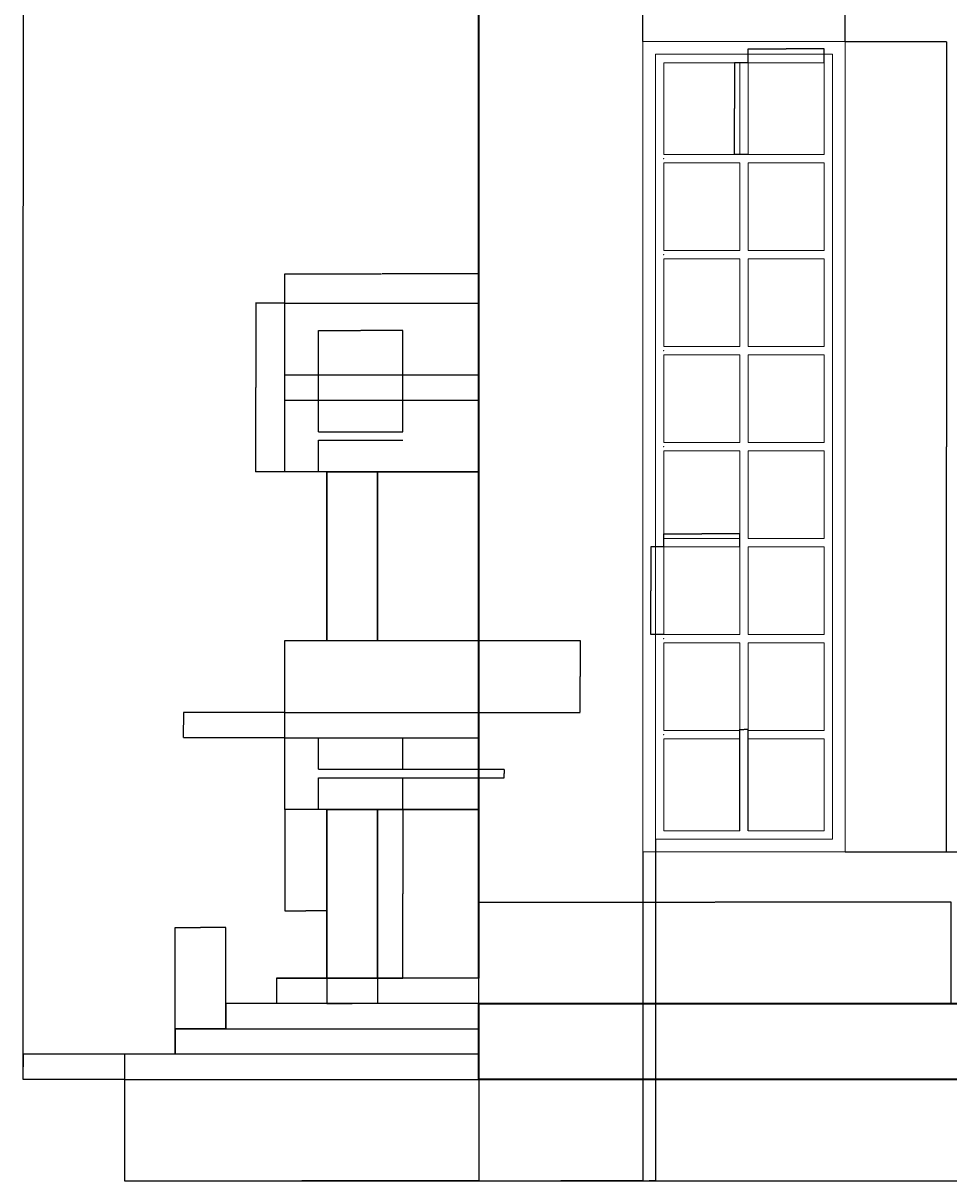
# Model space of a CAD drawing. Units: millimetres. Extents: x 54 to 12356, y 76 to 11627.
# Tile 1 of 2: x 54 to 5541, y 76 to 6935. Entities that reach past the tile are written whole.
import ezdxf

# ---------------------------------------------------------------- set-up
doc = ezdxf.new("R2010")
doc.units = ezdxf.units.MM
for name, color, linetype, lineweight in [('A-ANNO-DIMS', 2, 'Continuous', 18), ('A-COLS', 7, 'Continuous', 30), ('A-FLOR', 7, 'Continuous', 25), ('A-FLOR-STRS', 7, 'Continuous', 25), ('A-GLAZ', 4, 'Continuous', 18), ('A-GLAZ-LAYO', 8, 'Continuous', 13), ('A-WALL', 7, 'Continuous', 35), ('S-FNDN', 7, 'Continuous', 35)]:
    doc.layers.add(name, color=color, linetype=linetype, lineweight=lineweight)
doc.styles.get("Standard").update_dxf_attribs({"font": 'arial.ttf'})
doc.dimstyles.get("Standard").update_dxf_attribs({"dimtxt": 0.18, "dimasz": 0.18, "dimexe": 0.18, "dimexo": 0.0625, "dimgap": 0.09, "dimtad": 0, "dimtih": 1, "dimtoh": 1, "dimdec": 4, "dimzin": 0, "dimdsep": 46, "dimtxsty": 'Standard', "dimcen": 0.09, "dimadec": 0, "dimazin": 0, "dimtfac": 1, "dimtdec": 4, "dimtofl": 0, "dimtmove": 0, "dimatfit": 3, "dimfxl": 1, "dimtolj": 1, "dimtzin": 0, "dimarcsym": 0})

# ---------------------------------------------------------------- blocks, each defined once
blk = doc.blocks.new('STAIR-GLAZ-LITE-INTERMEDIATE')
for p, q in [((0.0003419131726332, 518.7501830437077), (450.0003419131708, 518.7501830437077)), ((0.0003419131726332, 0.0001830437076933), (0.000341913173088, 518.7501830437077)), ((450.0003419131717, 518.7501830437077), (450.0003419131726, 0.0001830437076933)), ((0.0003419131726332, 0.0001830437076933), (450.0003419131717, 0.0001830437076933))]:
    blk.add_line(p, q)
blk = doc.blocks.new('STAIR-GLAZ-LITE-END')
for p, q in [((0.0003419131726332, 543.7501830437077), (0.0003419131717237, 0.0001830437067838)), ((0.0003419131735427, 543.7501830437077), (450.0003419131726, 543.7501830437077)), ((450.0003419131726, 543.7501830437077), (450.0003419131726, 0.0001830437067838)), ((0.0003419131726332, 0.0001830437076933), (450.0003419131726, 0.0001830437076933))]:
    blk.add_line(p, q)
blk = doc.blocks.new('PORCH-COLUMN-300')
for p, q in [((0.0002773238852569, 0.0003573361398139), (0.0002773238852569, 1000.00035733614)), ((300.0002773238853, 0.0003573361398139), (300.0002773238853, 1000.00035733614))]:
    blk.add_line(p, q)
blk = doc.blocks.new('PORCH-FASCIA-1150')
for p, q in [((0.0002773238852569, 1000.00035733614), (1150.000277323885, 1000.00035733614)), ((0.0002773238852569, 575.00035733614), (0.0002773238852569, 1000.00035733614)), ((0.0002773238852569, 575.00035733614), (1150.000277323885, 575.00035733614)), ((0.0002773238852569, 425.00035733614), (0.0002773238852569, 575.00035733614)), ((0.0002773238852569, 0.0003573361400413), (0.0002773238852569, 425.00035733614)), ((0.0002773238852569, 425.00035733614), (1150.000277323885, 425.00035733614)), ((250.0002773238853, 0.0003573361400413), (0.0002773238852569, 0.0003573361400413)), ((250.0002773238853, 0.0003573361400413), (1150.000277323885, 0.0003573361400413)), ((1150.000277323885, 0.0003573361400413), (250.0002773238853, 0.0003573361400413))]:
    blk.add_line(p, q)
blk = doc.blocks.new('*D7')
at = {"layer": 'A-ANNO-DIMS', "color": 0, "lineweight": -2, "transparency": 16777216}
for p, q in [((3851.677841913175, 3831.536183043709), (3773.747841913177, 3831.536183043709)), ((3773.927841913176, 3831.356183043709), (3773.927841913176, 3572.343086181499)), ((3773.927841913176, 3312.966183043709), (3773.927841913176, 3571.97927990592)), ((3851.677841913175, 3312.786183043709), (3773.747841913177, 3312.786183043709))]:
    blk.add_line(p, q, dxfattribs=at)
at = {"layer": 'A-ANNO-DIMS', "color": 0, "transparency": 16777216}
for points in [[(3773.897841913176, 3831.356183043709), (3773.957841913177, 3831.356183043709), (3773.927841913176, 3831.536183043709)], [(3773.897841913176, 3312.966183043709), (3773.957841913177, 3312.966183043709), (3773.927841913176, 3312.786183043709)]]:
    blk.add_solid(points, dxfattribs=at)
at = {"layer": 'Defpoints', "color": 0, "transparency": 16777216}
for p in [(3851.740341913174, 3831.536183043709), (3773.927841913176, 3312.786183043709), (3851.740341913174, 3312.786183043709)]:
    blk.add_point(p, dxfattribs=at)
at = {"layer": 'A-ANNO-DIMS', "color": 0, "transparency": 16777216, "insert": (3773.927841913176, 3572.161183043707), "char_height": 0.18, "attachment_point": 5}
blk.add_mtext('\\A1;INTERMEDIATE LITE 519 TYP.', dxfattribs=at)
blk = doc.blocks.new('*D8')
at = {"layer": 'A-ANNO-DIMS', "color": 0, "lineweight": -2, "transparency": 16777216}
for p, q in [((3851.740341913173, 3831.598683043708), (3851.740341913173, 3909.528683043708)), ((3851.920341913173, 3909.348683043707), (4076.138704805396, 3909.348683043707)), ((4301.560341913172, 3909.348683043707), (4077.341979020949, 3909.348683043707)), ((4301.740341913173, 3831.598683043708), (4301.740341913173, 3909.528683043708))]:
    blk.add_line(p, q, dxfattribs=at)
at = {"layer": 'A-ANNO-DIMS', "color": 0, "transparency": 16777216}
for points in [[(3851.920341913173, 3909.378683043708), (3851.920341913173, 3909.318683043707), (3851.740341913173, 3909.348683043707)], [(4301.560341913172, 3909.378683043708), (4301.560341913172, 3909.318683043707), (4301.740341913173, 3909.348683043707)]]:
    blk.add_solid(points, dxfattribs=at)
at = {"layer": 'Defpoints', "color": 0, "transparency": 16777216}
for p in [(3851.740341913173, 3909.348683043707), (3851.740341913173, 3831.536183043708), (4301.740341913173, 3831.536183043708)]:
    blk.add_point(p, dxfattribs=at)
at = {"layer": 'A-ANNO-DIMS', "color": 0, "transparency": 16777216, "insert": (4076.740341913172, 3909.348683043707), "char_height": 0.18, "attachment_point": 5}
blk.add_mtext('\\A1;450 TYP.', dxfattribs=at)
blk = doc.blocks.new('*D9')
at = {"layer": 'A-ANNO-DIMS', "color": 0, "lineweight": -2, "transparency": 16777216}
for p, q in [((4351.677841913173, 6700.286183043711), (4269.997841913174, 6700.286183043711)), ((4270.177841913175, 6700.106183043711), (4270.177841913175, 6428.592717832252)), ((4270.177841913175, 6156.716183043711), (4270.177841913175, 6428.229648255172)), ((4351.677841913173, 6156.53618304371), (4269.997841913174, 6156.53618304371))]:
    blk.add_line(p, q, dxfattribs=at)
at = {"layer": 'A-ANNO-DIMS', "color": 0, "transparency": 16777216}
for points in [[(4270.147841913175, 6700.106183043711), (4270.207841913175, 6700.106183043711), (4270.177841913175, 6700.286183043711)], [(4270.147841913175, 6156.716183043711), (4270.207841913175, 6156.716183043711), (4270.177841913175, 6156.53618304371)]]:
    blk.add_solid(points, dxfattribs=at)
at = {"layer": 'Defpoints', "color": 0, "transparency": 16777216}
for p in [(4270.177841913175, 6700.286183043711), (4351.740341913173, 6700.286183043711), (4351.740341913173, 6156.53618304371)]:
    blk.add_point(p, dxfattribs=at)
at = {"layer": 'A-ANNO-DIMS', "color": 0, "transparency": 16777216, "insert": (4270.177841913176, 6428.411183043708), "char_height": 0.18, "attachment_point": 5}
blk.add_mtext('\\A1;END LITE 544 TYP.', dxfattribs=at)
blk = doc.blocks.new('*D10')
at = {"layer": 'A-ANNO-DIMS', "color": 0, "lineweight": -2, "transparency": 16777216}
for p, q in [((4351.740341913171, 6700.348683043708), (4351.740341913171, 6782.028683043709)), ((4351.920341913172, 6781.848683043708), (4576.138704805394, 6781.848683043708)), ((4801.560341913172, 6781.848683043708), (4577.341979020948, 6781.848683043708)), ((4801.740341913173, 6700.348683043708), (4801.740341913173, 6782.028683043709))]:
    blk.add_line(p, q, dxfattribs=at)
at = {"layer": 'A-ANNO-DIMS', "color": 0, "transparency": 16777216}
for points in [[(4351.920341913172, 6781.878683043707), (4351.920341913172, 6781.818683043709), (4351.740341913171, 6781.848683043708)], [(4801.560341913172, 6781.878683043707), (4801.560341913172, 6781.818683043709), (4801.740341913173, 6781.848683043708)]]:
    blk.add_solid(points, dxfattribs=at)
at = {"layer": 'Defpoints', "color": 0, "transparency": 16777216}
for p in [(4801.740341913173, 6781.848683043708), (4351.740341913171, 6700.286183043708), (4801.740341913173, 6700.286183043708)]:
    blk.add_point(p, dxfattribs=at)
at = {"layer": 'A-ANNO-DIMS', "color": 0, "transparency": 16777216, "insert": (4576.740341913171, 6781.848683043708), "char_height": 0.18, "attachment_point": 5}
blk.add_mtext('\\A1;450 TYP.', dxfattribs=at)
blk = doc.blocks.new('*D15')
at = {"layer": 'A-ANNO-DIMS', "color": 0, "lineweight": -2, "transparency": 16777216}
for p, q in [((2154.993777323886, 2276.423357336141), (2305.111277323887, 2276.423357336141)), ((2304.931277323887, 2276.243357336141), (2304.931277323887, 1776.606488304763)), ((2304.931277323887, 1276.60335733614), (2304.931277323887, 1776.240226367518)), ((2154.993777323886, 1276.42335733614), (2305.111277323887, 1276.42335733614))]:
    blk.add_line(p, q, dxfattribs=at)
at = {"layer": 'A-ANNO-DIMS', "color": 0, "transparency": 16777216}
for points in [[(2304.901277323887, 2276.243357336141), (2304.961277323887, 2276.243357336141), (2304.931277323887, 2276.423357336141)], [(2304.901277323887, 1276.60335733614), (2304.961277323887, 1276.60335733614), (2304.931277323887, 1276.42335733614)]]:
    blk.add_solid(points, dxfattribs=at)
at = {"layer": 'Defpoints', "color": 0, "transparency": 16777216}
for p in [(2154.931277323886, 2276.423357336141), (2304.931277323887, 2276.423357336141), (2154.931277323886, 1276.42335733614)]:
    blk.add_point(p, dxfattribs=at)
at = {"layer": 'A-ANNO-DIMS', "color": 0, "transparency": 16777216, "insert": (2304.931277323887, 1776.423357336139), "char_height": 0.18, "attachment_point": 5}
blk.add_mtext('\\A1;PORCH COLUMN 1000 TYP.', dxfattribs=at)
blk = doc.blocks.new('*D16')
at = {"layer": 'A-ANNO-DIMS', "color": 0, "lineweight": -2, "transparency": 16777216}
for p, q in [((1854.931277323885, 1276.36085733614), (1854.931277323885, 1126.243357336139)), ((2154.931277323886, 1276.36085733614), (2154.931277323886, 1126.243357336139)), ((1855.111277323885, 1126.42335733614), (2004.333323708606, 1126.42335733614)), ((2154.751277323885, 1126.42335733614), (2005.529230939165, 1126.42335733614))]:
    blk.add_line(p, q, dxfattribs=at)
at = {"layer": 'A-ANNO-DIMS', "color": 0, "transparency": 16777216}
for points in [[(1855.111277323885, 1126.453357336139), (1855.111277323885, 1126.39335733614), (1854.931277323885, 1126.42335733614)], [(2154.751277323885, 1126.453357336139), (2154.751277323885, 1126.39335733614), (2154.931277323886, 1126.42335733614)]]:
    blk.add_solid(points, dxfattribs=at)
at = {"layer": 'Defpoints', "color": 0, "transparency": 16777216}
for p in [(1854.931277323885, 1276.42335733614), (2154.931277323886, 1276.42335733614), (2154.931277323886, 1126.42335733614)]:
    blk.add_point(p, dxfattribs=at)
at = {"layer": 'A-ANNO-DIMS', "color": 0, "transparency": 16777216, "insert": (2004.931277323885, 1126.42335733614), "char_height": 0.18, "attachment_point": 5}
blk.add_mtext('\\A1;300 TYP.', dxfattribs=at)
blk = doc.blocks.new('*D17')
at = {"layer": 'A-ANNO-DIMS', "color": 0, "lineweight": -2, "transparency": 16777216}
for p, q in [((1604.931277323885, 5276.48585733614), (1604.931277323885, 5449.10335733614)), ((1605.111277323885, 5448.923357336139), (2178.289790284322, 5448.923357336139)), ((2754.751277323885, 5448.923357336139), (2181.572764363449, 5448.923357336139)), ((2754.931277323886, 5276.48585733614), (2754.931277323886, 5449.10335733614))]:
    blk.add_line(p, q, dxfattribs=at)
at = {"layer": 'A-ANNO-DIMS', "color": 0, "transparency": 16777216}
for points in [[(1605.111277323885, 5448.95335733614), (1605.111277323885, 5448.89335733614), (1604.931277323885, 5448.923357336139)], [(2754.751277323885, 5448.95335733614), (2754.751277323885, 5448.89335733614), (2754.931277323886, 5448.923357336139)]]:
    blk.add_solid(points, dxfattribs=at)
at = {"layer": 'Defpoints', "color": 0, "transparency": 16777216}
for p in [(2754.931277323886, 5448.923357336139), (1604.931277323885, 5276.42335733614), (2754.931277323886, 5276.42335733614)]:
    blk.add_point(p, dxfattribs=at)
at = {"layer": 'A-ANNO-DIMS', "color": 0, "transparency": 16777216, "insert": (2179.931277323885, 5448.923357336139), "char_height": 0.18, "attachment_point": 5}
blk.add_mtext('\\A1;PORCH FASCIA 1150 TYP.', dxfattribs=at)
blk = doc.blocks.new('*D18')
at = {"layer": 'A-ANNO-DIMS', "color": 0, "lineweight": -2, "transparency": 16777216}
for p, q in [((1604.868777323886, 5276.423357336142), (1432.251277323886, 5276.423357336142)), ((1432.431277323886, 5276.243357336142), (1432.431277323886, 4776.605260473931)), ((1432.431277323886, 4276.603357336141), (1432.431277323886, 4776.241454198351)), ((1604.868777323886, 4276.423357336141), (1432.251277323886, 4276.423357336141))]:
    blk.add_line(p, q, dxfattribs=at)
at = {"layer": 'A-ANNO-DIMS', "color": 0, "transparency": 16777216}
for points in [[(1432.401277323886, 5276.243357336142), (1432.461277323886, 5276.243357336142), (1432.431277323886, 5276.423357336142)], [(1432.401277323886, 4276.603357336141), (1432.461277323886, 4276.603357336141), (1432.431277323886, 4276.423357336141)]]:
    blk.add_solid(points, dxfattribs=at)
at = {"layer": 'Defpoints', "color": 0, "transparency": 16777216}
for p in [(1432.431277323886, 5276.423357336142), (1604.931277323886, 5276.423357336142), (1604.931277323886, 4276.423357336141)]:
    blk.add_point(p, dxfattribs=at)
at = {"layer": 'A-ANNO-DIMS', "color": 0, "transparency": 16777216, "insert": (1432.431277323887, 4776.423357336141), "char_height": 0.18, "attachment_point": 5}
blk.add_mtext('\\A1;1000 TYP.', dxfattribs=at)
blk = doc.blocks.new('*D19')
at = {"layer": 'A-ANNO-DIMS', "color": 0, "lineweight": -2, "transparency": 16777216}
for p, q in [((654.931277, 676.360857), (654.931277, 75.74335700000005)), ((11754.931277, 676.360857), (11754.931277, 75.74335700000005)), ((655.1112769999999, 75.923357), (6204.511358855389, 75.923357)), ((11754.751277, 75.923357), (6205.351195144611, 75.923357))]:
    blk.add_line(p, q, dxfattribs=at)
at = {"layer": 'A-ANNO-DIMS', "color": 0, "transparency": 16777216}
for points in [[(655.1112769999999, 75.953357), (655.1112769999999, 75.893357), (654.931277, 75.923357)], [(11754.751277, 75.953357), (11754.751277, 75.893357), (11754.931277, 75.923357)]]:
    blk.add_solid(points, dxfattribs=at)
at = {"layer": 'Defpoints', "color": 0, "transparency": 16777216}
for p in [(654.931277, 676.423357), (11754.931277, 676.423357), (11754.931277, 75.923357)]:
    blk.add_point(p, dxfattribs=at)
at = {"layer": 'A-ANNO-DIMS', "color": 0, "transparency": 16777216, "insert": (6204.931277, 75.923357), "char_height": 0.18, "attachment_point": 5}
blk.add_mtext('\\A1;11100', dxfattribs=at)
blk = doc.blocks.new('*D20')
at = {"layer": 'A-ANNO-DIMS', "color": 0, "lineweight": -2, "transparency": 16777216}
for p, q in [((2379.868777000001, 11026.423357), (54.25127699999922, 11026.423357)), ((54.43127699999891, 11026.243357), (54.43127700000006, 5851.605321529333)), ((54.43127700000121, 676.6033570000001), (54.43127700000006, 5851.24139247067)), ((654.8687770000003, 676.4233570000002), (54.2512770000013, 676.4233570000001))]:
    blk.add_line(p, q, dxfattribs=at)
at = {"layer": 'A-ANNO-DIMS', "color": 0, "transparency": 16777216}
for points in [[(54.40127699999891, 11026.243357), (54.46127699999891, 11026.243357), (54.43127699999891, 11026.423357)], [(54.40127700000121, 676.6033570000001), (54.46127700000121, 676.6033570000001), (54.43127700000121, 676.4233570000001)]]:
    blk.add_solid(points, dxfattribs=at)
at = {"layer": 'Defpoints', "color": 0, "transparency": 16777216}
for p in [(54.43127699999891, 11026.423357), (2379.931277000001, 11026.423357), (654.9312770000003, 676.4233570000002)]:
    blk.add_point(p, dxfattribs=at)
at = {"layer": 'A-ANNO-DIMS', "color": 0, "transparency": 16777216, "insert": (54.4312770000017, 5851.423357000001), "char_height": 0.18, "attachment_point": 5}
blk.add_mtext('\\A1;10350', dxfattribs=at)
blk = doc.blocks.new('*D24')
at = {"layer": 'A-ANNO-DIMS', "color": 0, "lineweight": -2, "transparency": 16777216}
for p, q in [((654.931277, 676.360857), (654.931277, 75.74335700000005)), ((2754.931277, 676.360857), (2754.931277, 75.74335700000005)), ((655.1112769999999, 75.923357), (1704.571277, 75.923357)), ((2754.751277, 75.923357), (1705.291277, 75.923357))]:
    blk.add_line(p, q, dxfattribs=at)
at = {"layer": 'A-ANNO-DIMS', "color": 0, "transparency": 16777216}
for points in [[(655.1112769999999, 75.953357), (655.1112769999999, 75.893357), (654.931277, 75.923357)], [(2754.751277, 75.953357), (2754.751277, 75.893357), (2754.931277, 75.923357)]]:
    blk.add_solid(points, dxfattribs=at)
at = {"layer": 'Defpoints', "color": 0, "transparency": 16777216}
for p in [(654.931277, 676.423357), (2754.931277, 676.423357), (654.931277, 75.923357)]:
    blk.add_point(p, dxfattribs=at)
at = {"layer": 'A-ANNO-DIMS', "color": 0, "transparency": 16777216, "insert": (1704.931277, 75.923357), "char_height": 0.18, "attachment_point": 5}
blk.add_mtext('\\A1;2100', dxfattribs=at)
blk = doc.blocks.new('*D25')
at = {"layer": 'A-ANNO-DIMS', "color": 0, "lineweight": -2, "transparency": 16777216}
for p, q in [((2754.931277, 1126.485857), (2754.931277, 1727.103357)), ((2755.111277, 1726.923357), (4154.571277, 1726.923357)), ((5554.751277, 1726.923357), (4155.291276999999, 1726.923357)), ((5554.931277, 1126.485857), (5554.931277, 1727.103357))]:
    blk.add_line(p, q, dxfattribs=at)
at = {"layer": 'A-ANNO-DIMS', "color": 0, "transparency": 16777216}
for points in [[(2755.111277, 1726.953357), (2755.111277, 1726.893356999999), (2754.931277, 1726.923357)], [(5554.751277, 1726.953357), (5554.751277, 1726.893356999999), (5554.931277, 1726.923357)]]:
    blk.add_solid(points, dxfattribs=at)
at = {"layer": 'Defpoints', "color": 0, "transparency": 16777216}
for p in [(5554.931277, 1726.923357), (2754.931277, 1126.423357), (5554.931277, 1126.423357)]:
    blk.add_point(p, dxfattribs=at)
at = {"layer": 'A-ANNO-DIMS', "color": 0, "transparency": 16777216, "insert": (4154.931277, 1726.923357), "char_height": 0.18, "attachment_point": 5}
blk.add_mtext('\\A1;2800', dxfattribs=at)
blk = doc.blocks.new('*D34')
at = {"layer": 'A-ANNO-DIMS', "color": 0, "lineweight": -2, "transparency": 16777216}
for p, q in [((3726.740342, 2025.223683), (3726.740342, 75.74335699999983)), ((2754.931277, 1126.360857), (2754.931277, 75.74335699999983)), ((2755.111277, 75.923357), (3240.441921369032, 75.923357)), ((3726.560342000001, 75.923357), (3241.229697630969, 75.923357))]:
    blk.add_line(p, q, dxfattribs=at)
at = {"layer": 'A-ANNO-DIMS', "color": 0, "transparency": 16777216}
for points in [[(2755.111277, 75.953357), (2755.111277, 75.893357), (2754.931277, 75.923357)], [(3726.560342000001, 75.953357), (3726.560342000001, 75.893357), (3726.740342, 75.923357)]]:
    blk.add_solid(points, dxfattribs=at)
at = {"layer": 'Defpoints', "color": 0, "transparency": 16777216}
for p in [(3726.740342, 2025.286183), (2754.931277, 1126.423357), (3726.740342, 75.923357)]:
    blk.add_point(p, dxfattribs=at)
at = {"layer": 'A-ANNO-DIMS', "color": 0, "transparency": 16777216, "insert": (3240.8358095, 75.923357), "char_height": 0.18, "attachment_point": 5}
blk.add_mtext('\\A1;971.8', dxfattribs=at)
blk = doc.blocks.new('*D35')
at = {"layer": 'A-ANNO-DIMS', "color": 0, "lineweight": -2, "transparency": 16777216}
for p, q in [((3726.740342, 6825.348683), (3726.740342, 7425.966183000001)), ((3726.920342, 7425.786183000001), (4326.390348821282, 7425.786183000001)), ((4926.560342, 7425.786183000001), (4327.090335178717, 7425.786183000001)), ((4926.740342, 6825.348683), (4926.740342, 7425.966183000001))]:
    blk.add_line(p, q, dxfattribs=at)
at = {"layer": 'A-ANNO-DIMS', "color": 0, "transparency": 16777216}
for points in [[(3726.920342, 7425.816183000001), (3726.920342, 7425.756183), (3726.740342, 7425.786183000001)], [(4926.560342, 7425.816183000001), (4926.560342, 7425.756183), (4926.740342, 7425.786183000001)]]:
    blk.add_solid(points, dxfattribs=at)
at = {"layer": 'Defpoints', "color": 0, "transparency": 16777216}
for p in [(4926.740342, 7425.786183000001), (3726.740342, 6825.286183), (4926.740342, 6825.286183)]:
    blk.add_point(p, dxfattribs=at)
at = {"layer": 'A-ANNO-DIMS', "color": 0, "transparency": 16777216, "insert": (4326.740341999999, 7425.786183000001), "char_height": 0.18, "attachment_point": 5}
blk.add_mtext('\\A1;1200', dxfattribs=at)
blk = doc.blocks.new('*D36')
at = {"layer": 'A-ANNO-DIMS', "color": 0, "lineweight": -2, "transparency": 16777216}
for p, q in [((4926.802842000002, 6825.286183000004), (5527.420342000003, 6825.286183000004)), ((5527.240342000003, 6825.106183000004), (5527.240342000004, 4425.468086137792)), ((5527.240342000005, 2025.466183000001), (5527.240342000004, 4425.104279862212)), ((4926.802842000002, 2025.286183000001), (5527.420342000005, 2025.286183000001))]:
    blk.add_line(p, q, dxfattribs=at)
at = {"layer": 'A-ANNO-DIMS', "color": 0, "transparency": 16777216}
for points in [[(5527.210342000003, 6825.106183000004), (5527.270342000003, 6825.106183000004), (5527.240342000003, 6825.286183000004)], [(5527.210342000005, 2025.466183000001), (5527.270342000004, 2025.466183000001), (5527.240342000005, 2025.286183000001)]]:
    blk.add_solid(points, dxfattribs=at)
at = {"layer": 'Defpoints', "color": 0, "transparency": 16777216}
for p in [(4926.740342000002, 6825.286183000004), (4926.740342000002, 2025.286183000001), (5527.240342000005, 2025.286183000001)]:
    blk.add_point(p, dxfattribs=at)
at = {"layer": 'A-ANNO-DIMS', "color": 0, "transparency": 16777216, "insert": (5527.240342000004, 4425.286182999999), "char_height": 0.18, "attachment_point": 5}
blk.add_mtext('\\A1;4800', dxfattribs=at)
blk = doc.blocks.new('*D37')
at = {"layer": 'A-ANNO-DIMS', "color": 0, "lineweight": -2, "transparency": 16777216}
for p, q in [((4926.802842000002, 2025.286183000001), (12355.61127700001, 2025.286183000002)), ((12355.43127700001, 2025.106183000002), (12355.43127700001, 1576.036673137792)), ((12355.43127700001, 1126.603357000002), (12355.43127700001, 1575.672866862212)), ((2754.993777000001, 1126.423357), (12355.61127700001, 1126.423357000001))]:
    blk.add_line(p, q, dxfattribs=at)
at = {"layer": 'A-ANNO-DIMS', "color": 0, "transparency": 16777216}
for points in [[(12355.40127700001, 2025.106183000002), (12355.46127700001, 2025.106183000002), (12355.43127700001, 2025.286183000002)], [(12355.40127700001, 1126.603357000002), (12355.46127700001, 1126.603357000002), (12355.43127700001, 1126.423357000001)]]:
    blk.add_solid(points, dxfattribs=at)
at = {"layer": 'Defpoints', "color": 0, "transparency": 16777216}
for p in [(4926.740342000002, 2025.286183000001), (12355.43127700001, 2025.286183000002), (2754.931277000001, 1126.423357)]:
    blk.add_point(p, dxfattribs=at)
at = {"layer": 'A-ANNO-DIMS', "color": 0, "transparency": 16777216, "insert": (12355.43127700001, 1575.854769999998), "char_height": 0.18, "attachment_point": 5}
blk.add_mtext('\\A1;898.9', dxfattribs=at)
blk = doc.blocks.new('*D44')
at = {"layer": 'A-ANNO-DIMS', "color": 0, "lineweight": -2, "transparency": 16777216}
for p, q in [((954.931277, 976.4858569999999), (954.931277, 1577.103357)), ((955.1112769999999, 1576.923357), (1104.642798145975, 1576.923357)), ((1254.751277, 1576.923357), (1105.219755854024, 1576.923357)), ((1254.931277, 976.4858569999999), (1254.931277, 1577.103357))]:
    blk.add_line(p, q, dxfattribs=at)
at = {"layer": 'A-ANNO-DIMS', "color": 0, "transparency": 16777216}
for points in [[(955.1112769999999, 1576.953357), (955.1112769999999, 1576.893357), (954.931277, 1576.923357)], [(1254.751277, 1576.953357), (1254.751277, 1576.893357), (1254.931277, 1576.923357)]]:
    blk.add_solid(points, dxfattribs=at)
at = {"layer": 'Defpoints', "color": 0, "transparency": 16777216}
for p in [(1254.931277, 1576.923357), (954.931277, 976.423357), (1254.931277, 976.423357)]:
    blk.add_point(p, dxfattribs=at)
at = {"layer": 'A-ANNO-DIMS', "color": 0, "transparency": 16777216, "insert": (1104.931277, 1576.923357), "char_height": 0.18, "attachment_point": 5}
blk.add_mtext('\\A1;300', dxfattribs=at)
blk = doc.blocks.new('*D45')
at = {"layer": 'A-ANNO-DIMS', "color": 0, "lineweight": -2, "transparency": 16777216}
for p, q in [((654.8687770000003, 826.4233570000005), (54.25127700000013, 826.4233570000004)), ((54.43127700000004, 826.2433570000004), (54.43127700000006, 751.6052601377902)), ((54.43127700000007, 676.6033570000001), (54.43127700000006, 751.2414538622103)), ((654.8687770000003, 676.4233570000002), (54.25127700000016, 676.4233570000001))]:
    blk.add_line(p, q, dxfattribs=at)
at = {"layer": 'A-ANNO-DIMS', "color": 0, "transparency": 16777216}
for points in [[(54.40127700000004, 826.2433570000004), (54.46127700000004, 826.2433570000004), (54.43127700000004, 826.4233570000004)], [(54.40127700000007, 676.6033570000001), (54.46127700000007, 676.6033570000001), (54.43127700000007, 676.4233570000001)]]:
    blk.add_solid(points, dxfattribs=at)
at = {"layer": 'Defpoints', "color": 0, "transparency": 16777216}
for p in [(54.43127700000004, 826.4233570000004), (654.9312770000003, 826.4233570000005), (654.9312770000003, 676.4233570000002)]:
    blk.add_point(p, dxfattribs=at)
at = {"layer": 'A-ANNO-DIMS', "color": 0, "transparency": 16777216, "insert": (54.43127700000025, 751.4233570000001), "char_height": 0.18, "attachment_point": 5}
blk.add_mtext('\\A1;150', dxfattribs=at)
blk = doc.blocks.new('*D46')
at = {"layer": 'A-ANNO-DIMS', "color": 0, "lineweight": -2, "transparency": 16777216}
for p, q in [((1604.931277, 2276.360857), (1604.931277, 1675.743357)), ((1854.931277, 2276.360857), (1854.931277, 1675.743357)), ((1605.111277, 1675.923357), (1729.641201965893, 1675.923357)), ((1854.751277, 1675.923357), (1730.221352034106, 1675.923357))]:
    blk.add_line(p, q, dxfattribs=at)
at = {"layer": 'A-ANNO-DIMS', "color": 0, "transparency": 16777216}
for points in [[(1605.111277, 1675.953357), (1605.111277, 1675.893357), (1604.931277, 1675.923357)], [(1854.751277, 1675.953357), (1854.751277, 1675.893357), (1854.931277, 1675.923357)]]:
    blk.add_solid(points, dxfattribs=at)
at = {"layer": 'Defpoints', "color": 0, "transparency": 16777216}
for p in [(1604.931277, 2276.423357), (1854.931277, 2276.423357), (1604.931277, 1675.923357)]:
    blk.add_point(p, dxfattribs=at)
at = {"layer": 'A-ANNO-DIMS', "color": 0, "transparency": 16777216, "insert": (1729.931277, 1675.923357), "char_height": 0.18, "attachment_point": 5}
blk.add_mtext('\\A1;250', dxfattribs=at)
blk = doc.blocks.new('*D48')
at = {"layer": 'A-ANNO-DIMS', "color": 0, "lineweight": -2, "transparency": 16777216}
for p, q in [((3801.740342, 2100.223683), (3801.740342, 75.74335699999983)), ((3726.740342, 2025.223683), (3726.740342, 75.74335699999983)), ((3726.920342, 75.923357), (3764.021481154161, 75.923357)), ((3801.560342000001, 75.923357), (3764.459202845839, 75.923357))]:
    blk.add_line(p, q, dxfattribs=at)
at = {"layer": 'A-ANNO-DIMS', "color": 0, "transparency": 16777216}
for points in [[(3726.920342, 75.953357), (3726.920342, 75.893357), (3726.740342, 75.923357)], [(3801.560342000001, 75.953357), (3801.560342000001, 75.893357), (3801.740342, 75.923357)]]:
    blk.add_solid(points, dxfattribs=at)
at = {"layer": 'Defpoints', "color": 0, "transparency": 16777216}
for p in [(3801.740342, 2100.286183), (3726.740342, 2025.286183), (3801.740342, 75.923357)]:
    blk.add_point(p, dxfattribs=at)
at = {"layer": 'A-ANNO-DIMS', "color": 0, "transparency": 16777216, "insert": (3764.240342, 75.923357), "char_height": 0.18, "attachment_point": 5}
blk.add_mtext('\\A1;75', dxfattribs=at)
blk = doc.blocks.new('*D49')
at = {"layer": 'A-ANNO-DIMS', "color": 0, "lineweight": -2, "transparency": 16777216}
for p, q in [((4301.740342, 2150.348683), (4301.740342, 2750.966183)), ((4301.920342, 2750.786183000001), (4326.521726720327, 2750.786183000001)), ((4351.560341999999, 2750.786183000001), (4326.958957279673, 2750.786183000001)), ((4351.740342, 2150.348683), (4351.740342, 2750.966183))]:
    blk.add_line(p, q, dxfattribs=at)
at = {"layer": 'A-ANNO-DIMS', "color": 0, "transparency": 16777216}
for points in [[(4301.920342, 2750.816183000001), (4301.920342, 2750.756183), (4301.740342, 2750.786183000001)], [(4351.560341999999, 2750.816183000001), (4351.560341999999, 2750.756183), (4351.740342, 2750.786183000001)]]:
    blk.add_solid(points, dxfattribs=at)
at = {"layer": 'Defpoints', "color": 0, "transparency": 16777216}
for p in [(4351.740342, 2750.786183000001), (4301.740342, 2150.286183), (4351.740342, 2150.286183)]:
    blk.add_point(p, dxfattribs=at)
at = {"layer": 'A-ANNO-DIMS', "color": 0, "transparency": 16777216, "insert": (4326.740341999999, 2750.786183000001), "char_height": 0.18, "attachment_point": 5}
blk.add_mtext('\\A1;50', dxfattribs=at)
blk = doc.blocks.new('*D50')
at = {"layer": 'A-ANNO-DIMS', "color": 0, "lineweight": -2, "transparency": 16777216}
for p, q in [((1804.931277, 4513.985856999999), (1804.931277, 5114.603357)), ((1805.111277, 5114.423356999999), (2054.642736754434, 5114.423356999999)), ((2304.751277000001, 5114.423356999999), (2055.219817245566, 5114.423356999999)), ((2304.931277, 4513.985856999999), (2304.931277, 5114.603357))]:
    blk.add_line(p, q, dxfattribs=at)
at = {"layer": 'A-ANNO-DIMS', "color": 0, "transparency": 16777216}
for points in [[(1805.111277, 5114.453356999999), (1805.111277, 5114.393357), (1804.931277, 5114.423356999999)], [(2304.751277000001, 5114.453356999999), (2304.751277000001, 5114.393357), (2304.931277, 5114.423356999999)]]:
    blk.add_solid(points, dxfattribs=at)
at = {"layer": 'Defpoints', "color": 0, "transparency": 16777216}
for p in [(2304.931277, 5114.423356999999), (1804.931277, 4513.923356999999), (2304.931277, 4513.923356999999)]:
    blk.add_point(p, dxfattribs=at)
at = {"layer": 'A-ANNO-DIMS', "color": 0, "transparency": 16777216, "insert": (2054.931277, 5114.423356999999), "char_height": 0.18, "attachment_point": 5}
blk.add_mtext('\\A1;500', dxfattribs=at)
blk = doc.blocks.new('*D51')
at = {"layer": 'A-ANNO-DIMS', "color": 0, "lineweight": -2, "transparency": 16777216}
for p, q in [((1604.868777000001, 2851.423357000001), (1004.251277000001, 2851.423357000001)), ((1004.431277000001, 2851.243357000001), (1004.431277000001, 2776.605260137791)), ((1004.431277000001, 2701.603357000001), (1004.431277000001, 2776.241453862211)), ((1604.868777000001, 2701.423357000001), (1004.251277000001, 2701.423357000001))]:
    blk.add_line(p, q, dxfattribs=at)
at = {"layer": 'A-ANNO-DIMS', "color": 0, "transparency": 16777216}
for points in [[(1004.401277000001, 2851.243357000001), (1004.461277, 2851.243357000001), (1004.431277000001, 2851.423357000001)], [(1004.401277000001, 2701.603357000001), (1004.461277000001, 2701.603357000001), (1004.431277000001, 2701.423357000001)]]:
    blk.add_solid(points, dxfattribs=at)
at = {"layer": 'Defpoints', "color": 0, "transparency": 16777216}
for p in [(1004.431277000001, 2851.423357000001), (1604.931277000001, 2851.423357000001), (1604.931277000001, 2701.423357000001)]:
    blk.add_point(p, dxfattribs=at)
at = {"layer": 'A-ANNO-DIMS', "color": 0, "transparency": 16777216, "insert": (1004.431277000001, 2776.423357), "char_height": 0.18, "attachment_point": 5}
blk.add_mtext('\\A1;150', dxfattribs=at)
blk = doc.blocks.new('*D52')
at = {"layer": 'A-ANNO-DIMS', "color": 0, "lineweight": -2, "transparency": 16777216}
for p, q in [((2304.993777000001, 2513.923357000001), (2905.611277000002, 2513.923357000001)), ((2905.431277000002, 2513.743357000001), (2905.431277000002, 2489.105260137791)), ((2905.431277000002, 2464.103357000001), (2905.431277000002, 2488.741453862211)), ((2304.993777000001, 2463.923357000001), (2905.611277000002, 2463.923357000001))]:
    blk.add_line(p, q, dxfattribs=at)
at = {"layer": 'A-ANNO-DIMS', "color": 0, "transparency": 16777216}
for points in [[(2905.401277000002, 2513.743357000001), (2905.461277000002, 2513.743357000001), (2905.431277000002, 2513.923357000001)], [(2905.401277000002, 2464.103357000001), (2905.461277000002, 2464.103357000001), (2905.431277000002, 2463.923357000001)]]:
    blk.add_solid(points, dxfattribs=at)
at = {"layer": 'Defpoints', "color": 0, "transparency": 16777216}
for p in [(2304.931277000001, 2513.923357000001), (2304.931277000001, 2463.923357000001), (2905.431277000002, 2463.923357000001)]:
    blk.add_point(p, dxfattribs=at)
at = {"layer": 'A-ANNO-DIMS', "color": 0, "transparency": 16777216, "insert": (2905.431277000002, 2488.923357), "char_height": 0.18, "attachment_point": 5}
blk.add_mtext('\\A1;50', dxfattribs=at)
blk = doc.blocks.new('*D53')
at = {"layer": 'A-ANNO-DIMS', "color": 0, "lineweight": -2, "transparency": 16777216}
for p, q in [((2754.993777000001, 3276.423357000002), (3355.611277000003, 3276.423357000002)), ((3355.431277000003, 3276.243357000003), (3355.431277000004, 3064.105260137792)), ((3355.431277000004, 2851.603357000002), (3355.431277000004, 3063.741453862212)), ((2754.993777000001, 2851.423357000001), (3355.611277000003, 2851.423357000001))]:
    blk.add_line(p, q, dxfattribs=at)
at = {"layer": 'A-ANNO-DIMS', "color": 0, "transparency": 16777216}
for points in [[(3355.401277000003, 3276.243357000003), (3355.461277000003, 3276.243357000003), (3355.431277000003, 3276.423357000002)], [(3355.401277000004, 2851.603357000002), (3355.461277000004, 2851.603357000002), (3355.431277000004, 2851.423357000001)]]:
    blk.add_solid(points, dxfattribs=at)
at = {"layer": 'Defpoints', "color": 0, "transparency": 16777216}
for p in [(2754.931277000001, 3276.423357000002), (2754.931277000001, 2851.423357000001), (3355.431277000004, 2851.423357000001)]:
    blk.add_point(p, dxfattribs=at)
at = {"layer": 'A-ANNO-DIMS', "color": 0, "transparency": 16777216, "insert": (3355.431277000003, 3063.923357000001), "char_height": 0.18, "attachment_point": 5}
blk.add_mtext('\\A1;425', dxfattribs=at)

msp = doc.modelspace()

# ---------------------------------------------------------------- linework, layer by layer
at = {"layer": 'A-FLOR'}
for p, q in [((1804.931277323886, 4513.92335733614), (1804.931277323886, 4701.42335733614)), ((1804.931277323886, 4513.92335733614), (2304.931277323885, 4513.92335733614)), ((1804.931277323886, 4276.42335733614), (1804.931277323886, 4463.92335733614)), ((1804.931277323886, 4463.92335733614), (2304.931277323885, 4463.92335733614)), ((1854.931277323886, 4276.42335733614), (1804.931277323886, 4276.42335733614)), ((2154.931277323886, 4276.42335733614), (2304.931277323885, 4276.42335733614)), ((1804.931277323886, 2513.92335733614), (1804.931277323886, 2701.42335733614)), ((2304.931277323885, 2513.92335733614), (2304.931277323885, 2701.42335733614)), ((1804.931277323885, 2513.92335733614), (2304.931277323885, 2513.92335733614)), ((1804.931277323885, 2276.42335733614), (1804.931277323886, 2463.92335733614)), ((1804.931277323885, 2463.92335733614), (2304.931277323885, 2463.92335733614)), ((2304.931277323885, 2276.42335733614), (2304.931277323885, 2463.92335733614)), ((1854.931277323885, 2276.42335733614), (1804.931277323885, 2276.42335733614)), ((2154.931277323886, 2276.42335733614), (2304.931277323885, 2276.42335733614))]:
    msp.add_line(p, q, dxfattribs=at)
at = {"layer": 'A-FLOR-STRS'}
for p, q in [((2754.931277323886, 1276.42335733614), (1554.931277323885, 1276.42335733614)), ((1554.931277323885, 1276.42335733614), (1554.931277323885, 1126.42335733614)), ((1554.931277323885, 1276.42335733614), (1854.931277323885, 1276.42335733614)), ((1854.931277323885, 1276.42335733614), (2154.931277323886, 1276.42335733614)), ((2754.931277323886, 1126.42335733614), (2754.931277323886, 1276.42335733614)), ((1554.931277323885, 1126.42335733614), (1254.931277323885, 1126.42335733614)), ((1254.931277323885, 1126.42335733614), (1254.931277323885, 976.4233573361398)), ((2754.931277323886, 1126.42335733614), (1554.931277323885, 1126.42335733614)), ((2754.931277323886, 976.4233573361398), (2754.931277323886, 1126.42335733614)), ((1254.931277323885, 976.4233573361398), (954.9312773238852, 976.4233573361398)), ((954.9312773238852, 976.4233573361398), (954.9312773238852, 826.4233573361398)), ((954.9312773238852, 826.4233573361398), (954.9312773238852, 976.4233573361398)), ((954.9312773238852, 976.4233573361398), (2754.931277323886, 976.4233573361398)), ((954.9312773238852, 826.4233573361398), (654.9312773238852, 826.4233573361398)), ((654.9312773238852, 826.4233573361398), (654.9312773238852, 676.4233573361398)), ((2754.931277323886, 826.4233573361398), (954.9312773238852, 826.4233573361398)), ((2754.931277323886, 676.4233573361398), (2754.931277323886, 826.4233573361398)), ((654.9312773238852, 676.4233573361398), (2754.931277323886, 676.4233573361398))]:
    msp.add_line(p, q, dxfattribs=at)
at = {"layer": 'A-GLAZ'}
for p, q in [((3726.740341913173, 2025.286183043708), (3726.740341913173, 6825.286183043708)), ((3726.740341913173, 6825.286183043708), (4926.740341913173, 6825.286183043708)), ((3726.740341913173, 6825.286183043708), (3776.740341913173, 6825.286183043708)), ((3726.740341913173, 6825.286183043708), (3801.740341913173, 6825.286183043708)), ((4926.740341913173, 6825.286183043708), (4926.740341913173, 2025.286183043708)), ((3801.740341913173, 6750.286183043709), (3851.740341913173, 6750.286183043709)), ((4851.740341913172, 2100.286183043708), (4801.740341913173, 2100.286183043708)), ((4926.740341913173, 2025.286183043708), (3726.740341913173, 2025.286183043708)), ((4926.740341913173, 2025.286183043708), (4851.740341913172, 2025.286183043708))]:
    msp.add_line(p, q, dxfattribs=at)
msp.add_lwpolyline([(3801.740341913173, 6750.286183043709), (4851.740341913172, 6750.286183043709), (4851.740341913172, 2100.286183043708), (3801.740341913173, 2100.286183043708)], close=True, dxfattribs=at)
at = {"layer": 'A-GLAZ-LAYO'}
for p in [(3851.740341913173, 6131.536183043707), (3851.740341913173, 5562.786183043708), (3851.740341913173, 4994.036183043707), (3851.740341913173, 4425.286183043708), (3851.740341913173, 3856.536183043708), (3851.740341913173, 3287.786183043708), (3851.740341913173, 2719.036183043708)]:
    msp.add_point(p, dxfattribs=at)
at = {"layer": 'A-WALL'}
msp.add_line((2754.931277323886, 1276.42335733614), (2754.931277323885, 10226.42335733614), dxfattribs=at)
at = {"layer": 'S-FNDN'}
for p, q in [((2754.931277323886, 676.4233573361398), (2754.931277323886, 1126.42335733614)), ((2754.931277323886, 1126.42335733614), (11754.93127732388, 1126.42335733614)), ((4954.931277323885, 1126.42335733614), (5554.931277323885, 1126.42335733614)), ((11754.93127732388, 676.4233573361398), (2754.931277323886, 676.4233573361398))]:
    msp.add_line(p, q, dxfattribs=at)

# ---------------------------------------------------------------- block references
at = {"layer": 'A-COLS', "rotation": 180}
msp.add_blockref('PORCH-COLUMN-300', (2154.931554647771, 4276.423714672279), dxfattribs=at)
at = {"layer": 'A-COLS'}
msp.add_blockref('PORCH-COLUMN-300', (1854.931, 1276.423), dxfattribs=at)
at = {"layer": 'A-FLOR'}
for p in [(1604.931, 4276.423), (1604.931, 2276.423)]:
    msp.add_blockref('PORCH-FASCIA-1150', p, dxfattribs=at)
at = {"layer": 'A-GLAZ', "rotation": 180}
for name, p in [('STAIR-GLAZ-LITE-END', (4301.740683826344, 6700.286366087417)), ('STAIR-GLAZ-LITE-INTERMEDIATE', (4301.740683826345, 6106.536366087415)), ('STAIR-GLAZ-LITE-INTERMEDIATE', (4301.740683826346, 5537.786366087415)), ('STAIR-GLAZ-LITE-INTERMEDIATE', (4301.740683826345, 4969.036366087415)), ('STAIR-GLAZ-LITE-INTERMEDIATE', (4301.740683826345, 4400.286366087414)), ('STAIR-GLAZ-LITE-INTERMEDIATE', (4301.740683826345, 3831.536366087415)), ('STAIR-GLAZ-LITE-INTERMEDIATE', (4801.740683826345, 3262.786366087414))]:
    msp.add_blockref(name, p, dxfattribs=at)
at = {"layer": 'A-GLAZ'}
for name, p in [('STAIR-GLAZ-LITE-END', (4351.74, 6156.536)), ('STAIR-GLAZ-LITE-INTERMEDIATE', (4351.739999999998, 5587.786000000002)), ('STAIR-GLAZ-LITE-INTERMEDIATE', (4351.739999999997, 5019.036000000002)), ('STAIR-GLAZ-LITE-INTERMEDIATE', (4351.739999999998, 4450.286)), ('STAIR-GLAZ-LITE-INTERMEDIATE', (4351.739999999998, 3881.536000000001)), ('STAIR-GLAZ-LITE-INTERMEDIATE', (4351.739999999998, 3312.786000000001)), ('STAIR-GLAZ-LITE-INTERMEDIATE', (3851.74, 2744.036)), ('STAIR-GLAZ-LITE-END', (3851.74, 2150.285999999999)), ('STAIR-GLAZ-LITE-END', (4351.74, 2150.285999999999))]:
    msp.add_blockref(name, p, dxfattribs=at)

# ---------------------------------------------------------------- dimensions: what is measured, and where the dimension line sits
at = {"layer": 'A-ANNO-DIMS'}
for base, p1, p2, angle, override, picture, middle in [((54.43127699999891, 11026.423357), (654.931277, 676.423357), (2379.931277, 11026.423357), 90, {"dimdec": 0, "dimlfac": 1, "dimrnd": 0, "dimzin": 0, "dimdsep": 46, "dimlunit": 2}, '*D20', (54.4312770000017, 5851.423357000001)), ((5527.240342000005, 2025.286183000001), (4926.740342, 6825.286183), (4926.740342, 2025.286183), 270, {"dimdec": 0, "dimlfac": 1, "dimrnd": 0, "dimzin": 0, "dimdsep": 46, "dimlunit": 2}, '*D36', (5527.240342000004, 4425.286182999999)), ((3355.431277000004, 2851.423357000001), (2754.931277, 3276.423357), (2754.931277, 2851.423357), 270, {"dimdec": 0, "dimlfac": 1, "dimrnd": 0, "dimzin": 0, "dimdsep": 46, "dimlunit": 2}, '*D53', (3355.431277000003, 3063.923357000001)), ((1004.431277000001, 2851.423357000001), (1604.931277, 2701.423357), (1604.931277, 2851.423357), 90, {"dimdec": 0, "dimlfac": 1, "dimrnd": 0, "dimzin": 0, "dimdsep": 46, "dimlunit": 2}, '*D51', (1004.431277000001, 2776.423357)), ((2905.431277000002, 2463.923357000001), (2304.931277, 2513.923357), (2304.931277, 2463.923357), 270, {"dimdec": 0, "dimlfac": 1, "dimrnd": 0, "dimzin": 0, "dimdsep": 46, "dimlunit": 2}, '*D52', (2905.431277000002, 2488.923357)), ((1604.931277, 1675.923357), (1854.931277, 2276.423357), (1604.931277, 2276.423357), 180, {"dimdec": 0, "dimlfac": 1, "dimrnd": 0, "dimzin": 0, "dimdsep": 46, "dimlunit": 2}, '*D46', (1729.931277, 1675.923357)), ((12355.43127700001, 2025.286183000002), (2754.931277, 1126.423357), (4926.740342, 2025.286183), 90, {"dimdec": 1, "dimlfac": 1, "dimrnd": 0, "dimzin": 0, "dimdsep": 46, "dimlunit": 2}, '*D37', (12355.43127700001, 1575.854769999998)), ((54.43127700000004, 826.4233570000004), (654.931277, 676.423357), (654.931277, 826.423357), 90, {"dimdec": 0, "dimlfac": 1, "dimrnd": 0, "dimzin": 0, "dimdsep": 46, "dimlunit": 2}, '*D45', (54.43127700000025, 751.4233570000001))]:
    dim = msp.add_linear_dim(base=base, p1=p1, p2=p2, angle=angle, dimstyle='Standard', override=override, dxfattribs=at)
    dim.commit()
    dim.dimension.update_dxf_attribs({"geometry": picture, "text_midpoint": middle})
for base, p1, p2, override, picture, middle in [((4926.740342, 7425.786183000001), (3726.740342, 6825.286183), (4926.740342, 6825.286183), {"dimdec": 0, "dimlfac": 1, "dimrnd": 0, "dimzin": 0, "dimdsep": 46, "dimlunit": 2}, '*D35', (4326.740341999999, 7425.786183000001)), ((2304.931277, 5114.423356999999), (1804.931277, 4513.923356999999), (2304.931277, 4513.923356999999), {"dimdec": 0, "dimlfac": 1, "dimrnd": 0, "dimzin": 0, "dimdsep": 46, "dimlunit": 2}, '*D50', (2054.931277, 5114.423356999999)), ((4351.740342, 2750.786183000001), (4301.740342, 2150.286183), (4351.740342, 2150.286183), {"dimdec": 0, "dimlfac": 1, "dimrnd": 0, "dimzin": 0, "dimdsep": 46, "dimlunit": 2}, '*D49', (4326.740341999999, 2750.786183000001)), ((3801.740342, 75.923357), (3726.740342, 2025.286183), (3801.740342, 2100.286183), {"dimdec": 0, "dimlfac": 1, "dimrnd": 0, "dimzin": 0, "dimdsep": 46, "dimlunit": 2}, '*D48', (3764.240342, 75.923357)), ((3726.740342, 75.923357), (2754.931277, 1126.423357), (3726.740342, 2025.286183), {"dimdec": 1, "dimlfac": 1, "dimrnd": 0, "dimzin": 0, "dimdsep": 46, "dimlunit": 2}, '*D34', (3240.8358095, 75.923357)), ((5554.931277, 1726.923357), (2754.931277, 1126.423357), (5554.931277, 1126.423357), {"dimdec": 0, "dimlfac": 1, "dimrnd": 0, "dimzin": 0, "dimdsep": 46, "dimlunit": 2}, '*D25', (4154.931277, 1726.923357)), ((1254.931277, 1576.923357), (954.931277, 976.423357), (1254.931277, 976.423357), {"dimdec": 0, "dimlfac": 1, "dimrnd": 0, "dimzin": 0, "dimdsep": 46, "dimlunit": 2}, '*D44', (1104.931277, 1576.923357)), ((11754.931277, 75.923357), (654.931277, 676.423357), (11754.931277, 676.423357), {"dimdec": 0, "dimlfac": 1, "dimrnd": 0, "dimzin": 0, "dimdsep": 46, "dimlunit": 2}, '*D19', (6204.931277, 75.923357)), ((654.931277, 75.923357), (2754.931277, 676.423357), (654.931277, 676.423357), {"dimdec": 0, "dimlfac": 1, "dimrnd": 0, "dimzin": 0, "dimdsep": 46, "dimlunit": 2}, '*D24', (1704.931277, 75.923357))]:
    dim = msp.add_linear_dim(base=base, p1=p1, p2=p2, dimstyle='Standard', override=override, dxfattribs=at)
    dim.commit()
    dim.dimension.update_dxf_attribs({"geometry": picture, "text_midpoint": middle})
for base, p1, p2, text, picture, middle in [((4801.740341913173, 6781.848683043708), (4351.740341913171, 6700.286183043708), (4801.740341913173, 6700.286183043708), '<> TYP.', '*D10', (4576.740341913171, 6781.848683043708)), ((2754.931277323886, 5448.923357336139), (1604.931277323885, 5276.42335733614), (2754.931277323886, 5276.42335733614), 'PORCH FASCIA <> TYP.', '*D17', (2179.931277323885, 5448.923357336139)), ((2154.931277323886, 1126.42335733614), (1854.931277323885, 1276.42335733614), (2154.931277323886, 1276.42335733614), '<> TYP.', '*D16', (2004.931277323885, 1126.42335733614))]:
    dim = msp.add_linear_dim(base=base, p1=p1, p2=p2, text=text, dimstyle='Standard', override={"dimdec": 0, "dimlfac": 1, "dimrnd": 0, "dimzin": 0, "dimdsep": 46, "dimlunit": 2}, dxfattribs=at)
    dim.commit()
    dim.dimension.update_dxf_attribs({"geometry": picture, "text_midpoint": middle})
for base, p1, p2, angle, text, picture, middle in [((4270.177841913175, 6700.286183043711), (4351.740341913171, 6156.536183043707), (4351.740341913171, 6700.286183043708), 90, 'END LITE <> TYP.', '*D9', (4270.177841913176, 6428.411183043708)), ((1432.431277323886, 5276.423357336142), (1604.931277323885, 4276.42335733614), (1604.931277323885, 5276.42335733614), 90, '<> TYP.', '*D18', (1432.431277323887, 4776.423357336141)), ((3851.740341913173, 3909.348683043707), (4301.740341913173, 3831.536183043708), (3851.740341913173, 3831.536183043708), 180, '<> TYP.', '*D8', (4076.740341913172, 3909.348683043707)), ((3773.927841913176, 3312.786183043709), (3851.740341913173, 3831.536183043708), (3851.740341913173, 3312.786183043708), 270, 'INTERMEDIATE LITE <> TYP.', '*D7', (3773.927841913176, 3572.161183043707)), ((2304.931277323887, 2276.423357336141), (2154.931277323886, 1276.42335733614), (2154.931277323886, 2276.42335733614), 90, 'PORCH COLUMN <> TYP.', '*D15', (2304.931277323887, 1776.423357336139))]:
    dim = msp.add_linear_dim(base=base, p1=p1, p2=p2, angle=angle, text=text, dimstyle='Standard', override={"dimdec": 0, "dimlfac": 1, "dimrnd": 0, "dimzin": 0, "dimdsep": 46, "dimlunit": 2}, dxfattribs=at)
    dim.commit()
    dim.dimension.update_dxf_attribs({"geometry": picture, "text_midpoint": middle})

doc.saveas('drawing.dxf')
